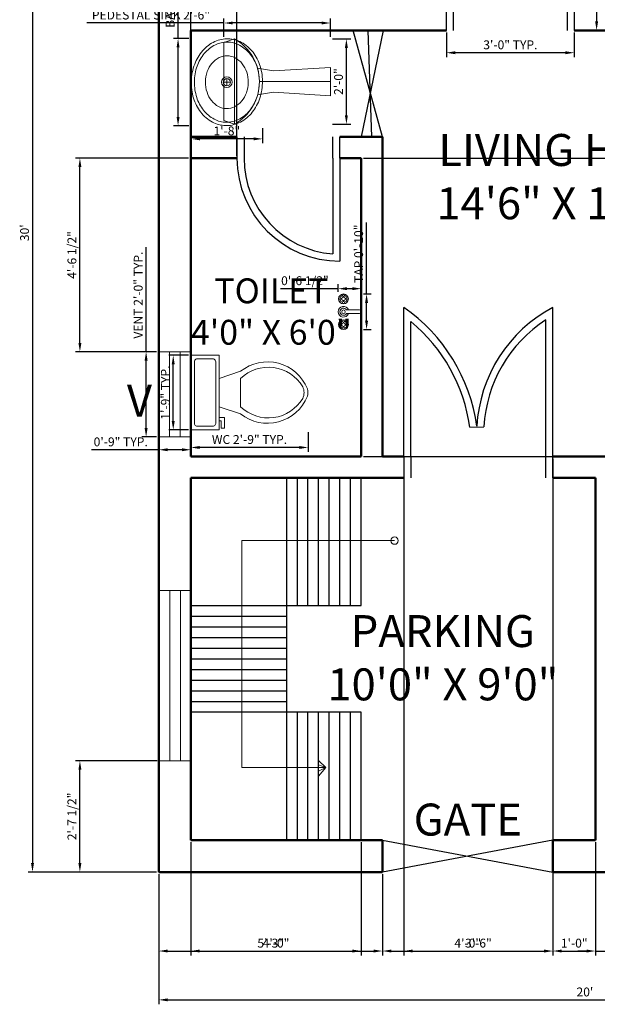
# Model space of a CAD drawing. Units: inches. Extents: x 2530 to 2846, y 1711 to 2145.
# Tile 1 of 3: x 2530 to 2693, y 1711 to 1989. Entities that reach past the tile are written whole.
import ezdxf

# ---------------------------------------------------------------- set-up
doc = ezdxf.new("R2010")
doc.units = ezdxf.units.IN
for name, color, linetype, lineweight in [('A-ANNO-DIMS', 2, 'Continuous', 18), ('A-ANNO-SYMB', 2, 'Continuous', 18), ('A-ANNO-TEXT', 7, 'Continuous', 18), ('A-AREA-IDEN', 7, 'Continuous', 25), ('A-DOOR', 3, 'Continuous', 25), ('A-FLOR-FIXT', 9, 'Continuous', 18), ('A-FLOR-STRS', 7, 'Continuous', 25), ('A-GLAZ', 4, 'Continuous', 18), ('A-WALL', 7, 'Continuous', 50)]:
    doc.layers.add(name, color=color, linetype=linetype, lineweight=lineweight)
doc.styles.get("Standard").update_dxf_attribs({"font": 'arial.ttf'})
doc.dimstyles.new('ISO-25', dxfattribs={"dimtxt": 2.5, "dimasz": 2.5, "dimexe": 1.25, "dimexo": 0.625, "dimtad": 1, "dimdec": 0, "dimlunit": 3, "dimtxsty": 'Standard', "dimcen": 2.5, "dimadec": 0, "dimazin": 0, "dimtfac": 1, "dimtdec": 0, "dimtmove": 0, "dimatfit": 3, "dimfxl": 1, "dimarcsym": 0})

# ---------------------------------------------------------------- blocks, each defined once
blk = doc.blocks.new('Faucet - Bathroom top')
for p, q in [((-4.107, 0.125), (-4.375, 0.125)), ((-3.75, 0.4788), (-3.75, 0.75)), ((-3.5, 0.482), (-3.5, 0.75)), ((-3.1461, 0.125), (-2.875, 0.125)), ((3.143, 0.125), (2.875, 0.125)), ((3.5, 0.4788), (3.5, 0.75)), ((3.75, 0.482), (3.75, 0.75)), ((4.1039, 0.125), (4.375, 0.125)), ((-4.1039, -0.125), (-4.375, -0.125)), ((-3.75, -0.4821), (-3.75, -0.75)), ((-3.5, -0.4789), (-3.5, -0.75)), ((-3.143, -0.125), (-2.875, -0.125)), ((-0.5, -0.8639), (-0.5, -4.5)), ((0.5, -4.5), (0.5, -0.8631)), ((3.1461, -0.125), (2.875, -0.125)), ((3.5, -0.4821), (3.5, -0.75)), ((3.75, -0.4789), (3.75, -0.75)), ((4.107, -0.125), (4.375, -0.125))]:
    blk.add_line(p, q)
for centre, radius in [((-3.625, 0), 1.375), ((-4.625, 0), 0.2795), ((-3.625, 0), 0.5), ((-3.625, 1), 0.2795), ((-2.625, 0), 0.2795), ((0, 0), 0.5), ((3.625, 0), 1.375), ((2.625, 0), 0.2795), ((3.625, 0), 0.5), ((3.625, 1), 0.2795), ((4.625, 0), 0.2795), ((-3.625, -1), 0.2795), ((3.625, -1), 0.2795)]:
    blk.add_circle(centre, radius)
for centre, radius, start, end in [((-3.625, 0), 1, 105.2407, 164.2093), ((-3.625, 0), 1, 16.44125, 74.07887), ((0, 0), 1.5, 289.6514, 250.3603), ((0, 0), 1, 300.3431, 239.7554), ((3.625, 0), 1, 106.12, 164.0884), ((3.625, 0), 1, 16.23422, 73.90469), ((-3.625, 0), 1, 196.2342, 253.9047), ((-3.625, 0), 1, 286.12, 344.0884), ((3.625, 0), 1, 196.4413, 254.0789), ((3.625, 0), 1, 285.2407, 344.2093), ((0, -4.5), 0.5, 180, 0)]:
    blk.add_arc(centre, radius, start, end)
blk = doc.blocks.new('Toilet - top')
for p, q in [((9.5, -6), (9.5, -2)), ((-8, -8.5), (-8, -8)), ((-7, -8), (-7, -9.5)), ((-4, -8), (-6, -14)), ((4, -8), (6, -14)), ((-10, -8.5), (-8, -8.5)), ((-10, -9.5), (-10, -8.5)), ((-7, -9.5), (-10, -9.5)), ((4, -14), (-4, -14))]:
    blk.add_line(p, q)
blk.add_lwpolyline([(10.5, -8), (10.5, 0), (-10.5, 0), (-10.5, -8)], close=True)
for points in [[(-9.5, -2), (-9.5, -6)], [(8.5, -1), (-8.5, -1)], [(-8.5, -7), (8.5, -7)]]:
    blk.add_lwpolyline(points)
for centre, radius, start, end in [((-8.62, -1.88), 0.884, 81.8699, 188.1301), ((8.62, -1.88), 0.884, 351.8699, 98.1301), ((-8.62, -6.12), 0.884, 171.8699, 278.1301), ((8.62, -6.12), 0.884, 261.8699, 8.1301), ((3.52, -21.58), 12.17, 141.4691, 247.9714), ((4.2, -21.82), 11.33, 136.3677, 238.9468), ((-3.52, -21.58), 12.17, 292.0284, 38.5307), ((-4.2, -21.82), 11.33, 301.053, 43.6321), ((0, -27.88), 4, 245.7318, 294.2682), ((0, -29), 4, 254.8605, 285.1395)]:
    blk.add_arc(centre, radius, start, end)
blk = doc.blocks.new('Sink - Oval top')
for p, q in [((-1, 0), (1, 0)), ((0, 1), (0, -1))]:
    blk.add_line(p, q)
for points in [[(-12.23, 0.39, 0.117634), (-11.46, -3.36, 0.104469), (-8.88, -6.8, 0.090016), (-5.08, -9.07, 0.08192), (-0.32, -10.02, 0.08192), (4.49, -9.38, 0.090016), (8.42, -7.36, 0.104469), (11.22, -4.09, 0.117634), (12.23, -0.39, 0.117634), (11.46, 3.36, 0.104469), (8.88, 6.8, 0.090016), (5.08, 9.07, 0.08192), (0.32, 10.02, 0.08192), (-4.49, 9.38, 0.090016), (-8.42, 7.36, 0.104469), (-11.22, 4.09, 0.117634)], [(-11.29, 0.16, 0.118622), (-10.52, -3.25, 0.104678), (-8.07, -6.36, 0.089562), (-4.54, -8.37, 0.081185), (-0.13, -9.15, 0.081185), (4.3, -8.49, 0.089562), (7.89, -6.58, 0.104678), (10.42, -3.55, 0.118622), (11.29, -0.16, 0.118622), (10.52, 3.25, 0.104678), (8.07, 6.36, 0.089562), (4.54, 8.37, 0.081185), (0.13, 9.15, 0.081185), (-4.3, 8.49, 0.089562), (-7.89, 6.58, 0.104678), (-10.42, 3.55, 0.118622)], [(-7.42, 0.08, 0.118283), (-6.91, -2.17, 0.104607), (-5.29, -4.21, 0.089718), (-2.97, -5.53, 0.081436), (-0.07, -6.04, 0.081436), (2.84, -5.59, 0.089718), (5.2, -4.33, 0.104607), (6.86, -2.32, 0.118283), (7.42, -0.08, 0.118283), (6.91, 2.17, 0.104607), (5.29, 4.21, 0.089718), (2.97, 5.53, 0.081436), (0.07, 6.04, 0.081436), (-2.84, 5.59, 0.089718), (-5.2, 4.33, 0.104607), (-6.86, 2.32, 0.118283)]]:
    blk.add_lwpolyline(points, format="xyb", close=True)
for radius in [1.5, 1]:
    blk.add_circle((0, 0), radius)
blk = doc.blocks.new('*D13')
at = {"layer": 'A-ANNO-DIMS', "color": 0, "lineweight": -2, "transparency": 16777216}
for p, q in [((2568.82, 2108.63), (2532.59, 2108.63)), ((2533.84, 2106.13), (2533.84, 1751.13)), ((2568.82, 1748.63), (2532.59, 1748.63))]:
    blk.add_line(p, q, dxfattribs=at)
at = {"layer": 'A-ANNO-DIMS', "color": 0, "transparency": 16777216}
for points in [[(2533.43, 2106.13), (2534.26, 2106.13), (2533.84, 2108.63)], [(2533.43, 1751.13), (2534.26, 1751.13), (2533.84, 1748.63)]]:
    blk.add_solid(points, dxfattribs=at)
at = {"layer": 'Defpoints', "color": 0, "transparency": 16777216}
for p in [(2569.45, 2108.63), (2533.84, 1748.63), (2569.45, 1748.63)]:
    blk.add_point(p, dxfattribs=at)
at = {"layer": 'A-ANNO-DIMS', "color": 0, "transparency": 16777216, "insert": (2531.94, 1928.63), "char_height": 2.5, "attachment_point": 5, "rotation": 90}
blk.add_mtext("30'", dxfattribs=at)
blk = doc.blocks.new('*D14')
at = {"layer": 'A-ANNO-DIMS', "color": 0, "lineweight": -2, "transparency": 16777216}
for p, q in [((2569.45, 1748), (2569.45, 1711.38)), ((2809.45, 1748), (2809.45, 1711.38)), ((2571.95, 1712.63), (2806.95, 1712.63))]:
    blk.add_line(p, q, dxfattribs=at)
at = {"layer": 'A-ANNO-DIMS', "color": 0, "transparency": 16777216}
for points in [[(2571.95, 1713.05), (2571.95, 1712.21), (2569.45, 1712.63)], [(2806.95, 1713.05), (2806.95, 1712.21), (2809.45, 1712.63)]]:
    blk.add_solid(points, dxfattribs=at)
at = {"layer": 'Defpoints', "color": 0, "transparency": 16777216}
for p in [(2569.45, 1748.63), (2809.45, 1748.63), (2809.45, 1712.63)]:
    blk.add_point(p, dxfattribs=at)
at = {"layer": 'A-ANNO-DIMS', "color": 0, "transparency": 16777216, "insert": (2689.45, 1714.53), "char_height": 2.5, "attachment_point": 5}
blk.add_mtext("20'", dxfattribs=at)
blk = doc.blocks.new('Sink - Pedestal elevation')
for p, q in [((-11, 30), (-12, 27)), ((-11, 30), (11, 30)), ((11, 30), (12, 27)), ((-12, 27), (12, 27)), ((-3, 16), (-3.7523, 20.5139)), ((0, 20), (0, 0)), ((3.7527, 20.5157), (3, 16)), ((-4, 0), (-3, 16)), ((3, 16), (4, 0)), ((-4, 0), (4, 0))]:
    blk.add_line(p, q)
blk.add_arc((0, 33.7857), 13.7857, 209.4871, 330.5129)
blk = doc.blocks.new('WIN-48IN')
for p, q in [((0, 48), (0, 0)), ((9, 48), (0, 48)), ((3, 48), (3, 0)), ((6, 0), (6, 48)), ((9, 0), (9, 48)), ((0, 0), (9, 0))]:
    blk.add_line(p, q)
blk = doc.blocks.new('VENT-24IN')
for p, q in [((24, 9), (0, 9)), ((0, 9), (0, 0)), ((24, 0), (24, 9)), ((24, 6), (0, 6)), ((0, 3), (24, 3)), ((0, 0), (24, 0))]:
    blk.add_line(p, q)
blk = doc.blocks.new('DOOR-SINGLE-29IN')
for p, q in [((0, 35), (0, 29)), ((2, 35), (2, 29)), ((27, 29), (27, 35)), ((29, 29), (29, 35)), ((27, 29), (27, 2.07)), ((29, 29), (29, 0))]:
    blk.add_line(p, q)
for radius, end in [(29, 270), (27, 265.752)]:
    blk.add_arc((29, 29), radius, 180, end)
blk = doc.blocks.new('DOOR-SINGLE-36IN')
for p, q in [((0, 36), (0, 42)), ((2, 36), (2, 42)), ((34, 42), (34, 36)), ((36, 42), (36, 36)), ((0, 36), (0, 0)), ((2, 36), (2, 2.06))]:
    blk.add_line(p, q)
for radius, start in [(36, 270), (34, 273.3723)]:
    blk.add_arc((0, 36), radius, start, 0)
blk = doc.blocks.new('*D24')
at = {"layer": 'A-ANNO-DIMS', "color": 0, "lineweight": -2, "transparency": 16777216}
for p, q in [((2578.45, 1872.51), (2578.45, 1866.92)), ((2611.49, 1872.51), (2611.49, 1866.92)), ((2608.99, 1868.17), (2580.95, 1868.17))]:
    blk.add_line(p, q, dxfattribs=at)
at = {"layer": 'A-ANNO-DIMS', "color": 0, "transparency": 16777216}
for points in [[(2580.95, 1868.59), (2580.95, 1867.76), (2578.45, 1868.17)], [(2608.99, 1868.59), (2608.99, 1867.76), (2611.49, 1868.17)]]:
    blk.add_solid(points, dxfattribs=at)
at = {"layer": 'Defpoints', "color": 0, "transparency": 16777216}
for p in [(2578.45, 1873.13), (2611.49, 1873.13), (2578.45, 1868.17)]:
    blk.add_point(p, dxfattribs=at)
at = {"layer": 'A-ANNO-DIMS', "color": 0, "transparency": 16777216, "insert": (2594.97, 1870.09), "char_height": 2.5, "attachment_point": 5}
blk.add_mtext('WC 2\'-9" TYP.', dxfattribs=at)
blk = doc.blocks.new('*D25')
at = {"layer": 'A-ANNO-DIMS', "color": 0, "lineweight": -2, "transparency": 16777216}
for p, q in [((2577.82, 1894.13), (2572.24, 1894.13)), ((2573.49, 1875.63), (2573.49, 1891.63)), ((2577.82, 1873.13), (2572.24, 1873.13))]:
    blk.add_line(p, q, dxfattribs=at)
at = {"layer": 'A-ANNO-DIMS', "color": 0, "transparency": 16777216}
for points in [[(2573.07, 1891.63), (2573.91, 1891.63), (2573.49, 1894.13)], [(2573.07, 1875.63), (2573.91, 1875.63), (2573.49, 1873.13)]]:
    blk.add_solid(points, dxfattribs=at)
at = {"layer": 'Defpoints', "color": 0, "transparency": 16777216}
for p in [(2573.49, 1894.13), (2578.45, 1894.13), (2578.45, 1873.13)]:
    blk.add_point(p, dxfattribs=at)
at = {"layer": 'A-ANNO-DIMS', "color": 0, "transparency": 16777216, "insert": (2571.59, 1883.63), "char_height": 2.5, "attachment_point": 5, "rotation": 90}
blk.add_mtext('1\'-9" TYP.', dxfattribs=at)
blk = doc.blocks.new('*D28')
at = {"layer": 'A-ANNO-DIMS', "color": 0, "lineweight": -2, "transparency": 16777216}
for p, q in [((2565.85, 1895.13), (2565.85, 1924.54)), ((2568.82, 1895.13), (2564.6, 1895.13)), ((2565.85, 1873.63), (2565.85, 1892.63)), ((2568.82, 1871.13), (2564.6, 1871.13))]:
    blk.add_line(p, q, dxfattribs=at)
at = {"layer": 'A-ANNO-DIMS', "color": 0, "transparency": 16777216}
for points in [[(2565.43, 1892.63), (2566.27, 1892.63), (2565.85, 1895.13)], [(2565.43, 1873.63), (2566.27, 1873.63), (2565.85, 1871.13)]]:
    blk.add_solid(points, dxfattribs=at)
at = {"layer": 'Defpoints', "color": 0, "transparency": 16777216}
for p in [(2565.85, 1895.13), (2569.45, 1895.13), (2569.45, 1871.13)]:
    blk.add_point(p, dxfattribs=at)
at = {"layer": 'A-ANNO-DIMS', "color": 0, "transparency": 16777216, "insert": (2563.95, 1911.08), "char_height": 2.5, "attachment_point": 5, "rotation": 90}
blk.add_mtext('VENT 2\'-0" TYP.', dxfattribs=at)
blk = doc.blocks.new('*D29')
at = {"layer": 'A-ANNO-DIMS', "color": 0, "lineweight": -2, "transparency": 16777216}
for p, q in [((2569.45, 1870.51), (2569.45, 1866.28)), ((2578.45, 1870.51), (2578.45, 1866.28)), ((2569.45, 1867.53), (2550.46, 1867.53)), ((2575.95, 1867.53), (2571.95, 1867.53))]:
    blk.add_line(p, q, dxfattribs=at)
at = {"layer": 'A-ANNO-DIMS', "color": 0, "transparency": 16777216}
for points in [[(2571.95, 1867.95), (2571.95, 1867.12), (2569.45, 1867.53)], [(2575.95, 1867.95), (2575.95, 1867.12), (2578.45, 1867.53)]]:
    blk.add_solid(points, dxfattribs=at)
at = {"layer": 'Defpoints', "color": 0, "transparency": 16777216}
for p in [(2569.45, 1871.13), (2578.45, 1871.13), (2569.45, 1867.53)]:
    blk.add_point(p, dxfattribs=at)
at = {"layer": 'A-ANNO-DIMS', "color": 0, "transparency": 16777216, "insert": (2558.7, 1869.43), "char_height": 2.5, "attachment_point": 5}
blk.add_mtext('0\'-9" TYP.', dxfattribs=at)
blk = doc.blocks.new('*D32')
at = {"layer": 'A-ANNO-DIMS', "color": 0, "lineweight": -2, "transparency": 16777216}
for p, q in [((2687.07, 2027.63), (2694, 2027.63)), ((2692.75, 2025.13), (2692.75, 1988.13)), ((2687.07, 1985.63), (2694, 1985.63))]:
    blk.add_line(p, q, dxfattribs=at)
at = {"layer": 'A-ANNO-DIMS', "color": 0, "transparency": 16777216}
for points in [[(2692.33, 2025.13), (2693.17, 2025.13), (2692.75, 2027.63)], [(2692.33, 1988.13), (2693.17, 1988.13), (2692.75, 1985.63)]]:
    blk.add_solid(points, dxfattribs=at)
at = {"layer": 'Defpoints', "color": 0, "transparency": 16777216}
for p in [(2686.45, 2027.63), (2686.45, 1985.63), (2692.75, 1985.63)]:
    blk.add_point(p, dxfattribs=at)
at = {"layer": 'A-ANNO-DIMS', "color": 0, "transparency": 16777216, "insert": (2690.83, 2006.63), "char_height": 2.5, "attachment_point": 5, "rotation": 90}
blk.add_mtext('DOOR 3\'-6" TYP.', dxfattribs=at)
blk = doc.blocks.new('*D33')
at = {"layer": 'A-ANNO-DIMS', "color": 0, "lineweight": -2, "transparency": 16777216}
for p, q in [((2650.45, 1985), (2650.45, 1978.08)), ((2686.45, 1985), (2686.45, 1978.08)), ((2683.95, 1979.33), (2652.95, 1979.33))]:
    blk.add_line(p, q, dxfattribs=at)
at = {"layer": 'A-ANNO-DIMS', "color": 0, "transparency": 16777216}
for points in [[(2652.95, 1979.75), (2652.95, 1978.91), (2650.45, 1979.33)], [(2683.95, 1979.75), (2683.95, 1978.91), (2686.45, 1979.33)]]:
    blk.add_solid(points, dxfattribs=at)
at = {"layer": 'Defpoints', "color": 0, "transparency": 16777216}
for p in [(2650.45, 1985.63), (2686.45, 1985.63), (2650.45, 1979.33)]:
    blk.add_point(p, dxfattribs=at)
at = {"layer": 'A-ANNO-DIMS', "color": 0, "transparency": 16777216, "insert": (2668.45, 1981.23), "char_height": 2.5, "attachment_point": 5}
blk.add_mtext('3\'-0" TYP.', dxfattribs=at)
blk = doc.blocks.new('*D34')
at = {"layer": 'A-ANNO-DIMS', "color": 0, "lineweight": -2, "transparency": 16777216}
for p, q in [((2627.95, 1911.39), (2627.95, 1931.55)), ((2627.07, 1911.39), (2629.2, 1911.39)), ((2627.95, 1903.89), (2627.95, 1908.89)), ((2627.07, 1901.39), (2629.2, 1901.39))]:
    blk.add_line(p, q, dxfattribs=at)
at = {"layer": 'A-ANNO-DIMS', "color": 0, "transparency": 16777216}
for points in [[(2627.53, 1908.89), (2628.37, 1908.89), (2627.95, 1911.39)], [(2627.53, 1903.89), (2628.37, 1903.89), (2627.95, 1901.39)]]:
    blk.add_solid(points, dxfattribs=at)
at = {"layer": 'Defpoints', "color": 0, "transparency": 16777216}
for p in [(2626.45, 1911.39), (2627.95, 1911.39), (2626.45, 1901.39)]:
    blk.add_point(p, dxfattribs=at)
at = {"layer": 'A-ANNO-DIMS', "color": 0, "transparency": 16777216, "insert": (2626.05, 1922.72), "char_height": 2.5, "attachment_point": 5, "rotation": 90}
blk.add_mtext('TAP 0\'-10"', dxfattribs=at)
blk = doc.blocks.new('*D35')
at = {"layer": 'A-ANNO-DIMS', "color": 0, "lineweight": -2, "transparency": 16777216}
for p, q in [((2619.95, 1912.01), (2619.95, 1914.14)), ((2626.45, 1912.01), (2626.45, 1914.14)), ((2619.95, 1912.89), (2603.73, 1912.89)), ((2623.95, 1912.89), (2622.45, 1912.89))]:
    blk.add_line(p, q, dxfattribs=at)
at = {"layer": 'A-ANNO-DIMS', "color": 0, "transparency": 16777216}
for points in [[(2622.45, 1913.31), (2622.45, 1912.47), (2619.95, 1912.89)], [(2623.95, 1913.31), (2623.95, 1912.47), (2626.45, 1912.89)]]:
    blk.add_solid(points, dxfattribs=at)
at = {"layer": 'Defpoints', "color": 0, "transparency": 16777216}
for p in [(2619.95, 1912.89), (2619.95, 1911.39), (2626.45, 1911.39)]:
    blk.add_point(p, dxfattribs=at)
at = {"layer": 'A-ANNO-DIMS', "color": 0, "transparency": 16777216, "insert": (2610.59, 1914.81), "char_height": 2.5, "attachment_point": 5}
blk.add_mtext('0\'-6 1/2"', dxfattribs=at)
blk = doc.blocks.new('*D44')
at = {"layer": 'A-ANNO-DIMS', "color": 0, "lineweight": -2, "transparency": 16777216}
for p, q in [((2574.85, 1983.31), (2574.85, 2010.87)), ((2577.91, 1983.31), (2573.6, 1983.31)), ((2574.85, 1961.26), (2574.85, 1980.81)), ((2577.91, 1958.76), (2573.6, 1958.76))]:
    blk.add_line(p, q, dxfattribs=at)
at = {"layer": 'A-ANNO-DIMS', "color": 0, "transparency": 16777216}
for points in [[(2574.43, 1980.81), (2575.27, 1980.81), (2574.85, 1983.31)], [(2574.43, 1961.26), (2575.27, 1961.26), (2574.85, 1958.76)]]:
    blk.add_solid(points, dxfattribs=at)
at = {"layer": 'Defpoints', "color": 0, "transparency": 16777216}
for p in [(2574.85, 1983.31), (2578.53, 1983.31), (2578.53, 1958.76)]:
    blk.add_point(p, dxfattribs=at)
at = {"layer": 'A-ANNO-DIMS', "color": 0, "transparency": 16777216, "insert": (2572.93, 1998.34), "char_height": 2.5, "attachment_point": 5, "rotation": 90}
blk.add_mtext('BASIN 2\'-0 1/2"', dxfattribs=at)
blk = doc.blocks.new('*D45')
at = {"layer": 'A-ANNO-DIMS', "color": 0, "lineweight": -2, "transparency": 16777216}
for p, q in [((2578.53, 1958.13), (2578.53, 1953.82)), ((2598.67, 1958.13), (2598.67, 1953.82)), ((2596.17, 1955.07), (2581.03, 1955.07))]:
    blk.add_line(p, q, dxfattribs=at)
at = {"layer": 'A-ANNO-DIMS', "color": 0, "transparency": 16777216}
for points in [[(2581.03, 1955.49), (2581.03, 1954.66), (2578.53, 1955.07)], [(2596.17, 1955.49), (2596.17, 1954.66), (2598.67, 1955.07)]]:
    blk.add_solid(points, dxfattribs=at)
at = {"layer": 'Defpoints', "color": 0, "transparency": 16777216}
for p in [(2578.53, 1958.76), (2598.67, 1958.76), (2578.53, 1955.07)]:
    blk.add_point(p, dxfattribs=at)
at = {"layer": 'A-ANNO-DIMS', "color": 0, "transparency": 16777216, "insert": (2588.6, 1956.98), "char_height": 2.5, "attachment_point": 5}
blk.add_mtext('1\'-8"', dxfattribs=at)
blk = doc.blocks.new('*D46')
at = {"layer": 'A-ANNO-DIMS', "color": 0, "lineweight": -2, "transparency": 16777216}
for p, q in [((2587.77, 1983.82), (2587.77, 1988.95)), ((2617.77, 1983.82), (2617.77, 1988.95)), ((2587.77, 1987.7), (2549.16, 1987.7)), ((2615.27, 1987.7), (2590.27, 1987.7))]:
    blk.add_line(p, q, dxfattribs=at)
at = {"layer": 'A-ANNO-DIMS', "color": 0, "transparency": 16777216}
for points in [[(2590.27, 1988.11), (2590.27, 1987.28), (2587.77, 1987.7)], [(2615.27, 1988.11), (2615.27, 1987.28), (2617.77, 1987.7)]]:
    blk.add_solid(points, dxfattribs=at)
at = {"layer": 'Defpoints', "color": 0, "transparency": 16777216}
for p in [(2587.77, 1987.7), (2587.77, 1983.2), (2617.77, 1983.2)]:
    blk.add_point(p, dxfattribs=at)
at = {"layer": 'A-ANNO-DIMS', "color": 0, "transparency": 16777216, "insert": (2567.21, 1989.62), "char_height": 2.5, "attachment_point": 5}
blk.add_mtext('PEDESTAL SINK 2\'-6"', dxfattribs=at)
blk = doc.blocks.new('*D47')
at = {"layer": 'A-ANNO-DIMS', "color": 0, "lineweight": -2, "transparency": 16777216}
for p, q in [((2618.39, 1983.2), (2623.52, 1983.2)), ((2622.27, 1961.7), (2622.27, 1980.7)), ((2618.39, 1959.2), (2623.52, 1959.2))]:
    blk.add_line(p, q, dxfattribs=at)
at = {"layer": 'A-ANNO-DIMS', "color": 0, "transparency": 16777216}
for points in [[(2621.85, 1980.7), (2622.68, 1980.7), (2622.27, 1983.2)], [(2621.85, 1961.7), (2622.68, 1961.7), (2622.27, 1959.2)]]:
    blk.add_solid(points, dxfattribs=at)
at = {"layer": 'Defpoints', "color": 0, "transparency": 16777216}
for p in [(2617.77, 1983.2), (2622.27, 1983.2), (2617.77, 1959.2)]:
    blk.add_point(p, dxfattribs=at)
at = {"layer": 'A-ANNO-DIMS', "color": 0, "transparency": 16777216, "insert": (2620.37, 1971.2), "char_height": 2.5, "attachment_point": 5, "rotation": 90}
blk.add_mtext('2\'-0"', dxfattribs=at)
blk = doc.blocks.new('*D48')
at = {"layer": 'A-ANNO-DIMS', "color": 0, "lineweight": -2, "transparency": 16777216}
for p, q in [((2569.45, 1748), (2569.45, 1725.13)), ((2632.45, 1748), (2632.45, 1725.13)), ((2571.95, 1726.38), (2629.95, 1726.38))]:
    blk.add_line(p, q, dxfattribs=at)
at = {"layer": 'A-ANNO-DIMS', "color": 0, "transparency": 16777216}
for points in [[(2571.95, 1726.8), (2571.95, 1725.96), (2569.45, 1726.38)], [(2629.95, 1726.8), (2629.95, 1725.96), (2632.45, 1726.38)]]:
    blk.add_solid(points, dxfattribs=at)
at = {"layer": 'Defpoints', "color": 0, "transparency": 16777216}
for p in [(2569.45, 1748.63), (2632.45, 1748.63), (2632.45, 1726.38)]:
    blk.add_point(p, dxfattribs=at)
at = {"layer": 'A-ANNO-DIMS', "color": 0, "transparency": 16777216, "insert": (2600.95, 1728.28), "char_height": 2.5, "attachment_point": 5}
blk.add_mtext('5\'-3"', dxfattribs=at)
blk = doc.blocks.new('*D49')
at = {"layer": 'A-ANNO-DIMS', "color": 0, "lineweight": -2, "transparency": 16777216}
for p, q in [((2632.45, 1748), (2632.45, 1725.13)), ((2680.45, 1748), (2680.45, 1725.13)), ((2634.95, 1726.38), (2677.95, 1726.38))]:
    blk.add_line(p, q, dxfattribs=at)
at = {"layer": 'A-ANNO-DIMS', "color": 0, "transparency": 16777216}
for points in [[(2634.95, 1726.8), (2634.95, 1725.96), (2632.45, 1726.38)], [(2677.95, 1726.8), (2677.95, 1725.96), (2680.45, 1726.38)]]:
    blk.add_solid(points, dxfattribs=at)
at = {"layer": 'Defpoints', "color": 0, "transparency": 16777216}
for p in [(2632.45, 1748.63), (2680.45, 1748.63), (2680.45, 1726.38)]:
    blk.add_point(p, dxfattribs=at)
at = {"layer": 'A-ANNO-DIMS', "color": 0, "transparency": 16777216, "insert": (2656.45, 1728.28), "char_height": 2.5, "attachment_point": 5}
blk.add_mtext('4\'-0"', dxfattribs=at)
blk = doc.blocks.new('*D50')
at = {"layer": 'A-ANNO-DIMS', "color": 0, "lineweight": -2, "transparency": 16777216}
for p, q in [((2692.45, 1757), (2692.45, 1725.13)), ((2680.45, 1748), (2680.45, 1725.13)), ((2682.95, 1726.38), (2689.95, 1726.38))]:
    blk.add_line(p, q, dxfattribs=at)
at = {"layer": 'A-ANNO-DIMS', "color": 0, "transparency": 16777216}
for points in [[(2682.95, 1726.8), (2682.95, 1725.96), (2680.45, 1726.38)], [(2689.95, 1726.8), (2689.95, 1725.96), (2692.45, 1726.38)]]:
    blk.add_solid(points, dxfattribs=at)
at = {"layer": 'Defpoints', "color": 0, "transparency": 16777216}
for p in [(2692.45, 1757.63), (2680.45, 1748.63), (2692.45, 1726.38)]:
    blk.add_point(p, dxfattribs=at)
at = {"layer": 'A-ANNO-DIMS', "color": 0, "transparency": 16777216, "insert": (2686.45, 1728.28), "char_height": 2.5, "attachment_point": 5}
blk.add_mtext('1\'-0"', dxfattribs=at)
blk = doc.blocks.new('*D51')
at = {"layer": 'A-ANNO-DIMS', "color": 0, "lineweight": -2, "transparency": 16777216}
for p, q in [((2638.45, 1865), (2638.45, 1725.13)), ((2680.45, 1865), (2680.45, 1725.13)), ((2640.95, 1726.38), (2677.95, 1726.38))]:
    blk.add_line(p, q, dxfattribs=at)
at = {"layer": 'A-ANNO-DIMS', "color": 0, "transparency": 16777216}
for points in [[(2640.95, 1726.8), (2640.95, 1725.96), (2638.45, 1726.38)], [(2677.95, 1726.8), (2677.95, 1725.96), (2680.45, 1726.38)]]:
    blk.add_solid(points, dxfattribs=at)
at = {"layer": 'Defpoints', "color": 0, "transparency": 16777216}
for p in [(2638.45, 1865.63), (2680.45, 1865.63), (2680.45, 1726.38)]:
    blk.add_point(p, dxfattribs=at)
at = {"layer": 'A-ANNO-DIMS', "color": 0, "transparency": 16777216, "insert": (2659.45, 1728.28), "char_height": 2.5, "attachment_point": 5}
blk.add_mtext('3\'-6"', dxfattribs=at)
blk = doc.blocks.new('*D57')
at = {"layer": 'A-ANNO-DIMS', "color": 0, "lineweight": -2, "transparency": 16777216}
for p, q in [((2692.45, 1757), (2692.45, 1725.13)), ((2698.45, 1757), (2698.45, 1725.13)), ((2689.95, 1726.38), (2687.45, 1726.38)), ((2692.45, 1726.38), (2698.45, 1726.38)), ((2700.95, 1726.38), (2711.34, 1726.38))]:
    blk.add_line(p, q, dxfattribs=at)
at = {"layer": 'A-ANNO-DIMS', "color": 0, "transparency": 16777216}
for points in [[(2689.95, 1726.8), (2689.95, 1725.96), (2692.45, 1726.38)], [(2700.95, 1726.8), (2700.95, 1725.96), (2698.45, 1726.38)]]:
    blk.add_solid(points, dxfattribs=at)
at = {"layer": 'Defpoints', "color": 0, "transparency": 16777216}
for p in [(2692.45, 1757.63), (2698.45, 1757.63), (2698.45, 1726.38)]:
    blk.add_point(p, dxfattribs=at)
at = {"layer": 'A-ANNO-DIMS', "color": 0, "transparency": 16777216, "insert": (2707.4, 1728.28), "char_height": 2.5, "attachment_point": 5}
blk.add_mtext('0\'-6"', dxfattribs=at)
blk = doc.blocks.new('*D58')
at = {"layer": 'A-ANNO-DIMS', "color": 0, "lineweight": -2, "transparency": 16777216}
for p, q in [((2627.07, 1949.63), (2832.95, 1949.63)), ((2831.7, 1868.13), (2831.7, 1947.13)), ((2627.07, 1865.63), (2832.95, 1865.63))]:
    blk.add_line(p, q, dxfattribs=at)
at = {"layer": 'A-ANNO-DIMS', "color": 0, "transparency": 16777216}
for points in [[(2831.28, 1947.13), (2832.12, 1947.13), (2831.7, 1949.63)], [(2831.28, 1868.13), (2832.12, 1868.13), (2831.7, 1865.63)]]:
    blk.add_solid(points, dxfattribs=at)
at = {"layer": 'Defpoints', "color": 0, "transparency": 16777216}
for p in [(2626.45, 1949.63), (2831.7, 1949.63), (2626.45, 1865.63)]:
    blk.add_point(p, dxfattribs=at)
at = {"layer": 'A-ANNO-DIMS', "color": 0, "transparency": 16777216, "insert": (2829.8, 1907.63), "char_height": 2.5, "attachment_point": 5, "rotation": 90}
blk.add_mtext('7\'-0"', dxfattribs=at)
blk = doc.blocks.new('*D63')
at = {"layer": 'A-ANNO-DIMS', "color": 0, "lineweight": -2, "transparency": 16777216}
for p, q in [((2568.95, 1779.94), (2545.95, 1779.94)), ((2547.2, 1751.13), (2547.2, 1777.44)), ((2568.82, 1748.63), (2545.95, 1748.63))]:
    blk.add_line(p, q, dxfattribs=at)
at = {"layer": 'A-ANNO-DIMS', "color": 0, "transparency": 16777216}
for points in [[(2546.78, 1777.44), (2547.62, 1777.44), (2547.2, 1779.94)], [(2546.78, 1751.13), (2547.62, 1751.13), (2547.2, 1748.63)]]:
    blk.add_solid(points, dxfattribs=at)
at = {"layer": 'Defpoints', "color": 0, "transparency": 16777216}
for p in [(2547.2, 1779.94), (2569.57, 1779.94), (2569.45, 1748.63)]:
    blk.add_point(p, dxfattribs=at)
at = {"layer": 'A-ANNO-DIMS', "color": 0, "transparency": 16777216, "insert": (2545.28, 1764.29), "char_height": 2.5, "attachment_point": 5, "rotation": 90}
blk.add_mtext('2\'-7 1/2"', dxfattribs=at)
blk = doc.blocks.new('*D67')
at = {"layer": 'A-ANNO-DIMS', "color": 0, "lineweight": -2, "transparency": 16777216}
for p, q in [((2578.45, 1757), (2578.45, 1725.13)), ((2626.45, 1757), (2626.45, 1725.13)), ((2580.95, 1726.38), (2623.95, 1726.38))]:
    blk.add_line(p, q, dxfattribs=at)
at = {"layer": 'A-ANNO-DIMS', "color": 0, "transparency": 16777216}
for points in [[(2580.95, 1726.8), (2580.95, 1725.96), (2578.45, 1726.38)], [(2623.95, 1726.8), (2623.95, 1725.96), (2626.45, 1726.38)]]:
    blk.add_solid(points, dxfattribs=at)
at = {"layer": 'Defpoints', "color": 0, "transparency": 16777216}
for p in [(2578.45, 1757.63), (2626.45, 1757.63), (2626.45, 1726.38)]:
    blk.add_point(p, dxfattribs=at)
at = {"layer": 'A-ANNO-DIMS', "color": 0, "transparency": 16777216, "insert": (2602.45, 1728.28), "char_height": 2.5, "attachment_point": 5}
blk.add_mtext('4\'-0"', dxfattribs=at)
blk = doc.blocks.new('*D68')
at = {"layer": 'A-ANNO-DIMS', "color": 0, "lineweight": -2, "transparency": 16777216}
for p, q in [((2578.45, 1950.25), (2578.45, 2132.13)), ((2591.45, 1950.25), (2591.45, 2132.13)), ((2580.95, 2130.88), (2588.95, 2130.88))]:
    blk.add_line(p, q, dxfattribs=at)
at = {"layer": 'A-ANNO-DIMS', "color": 0, "transparency": 16777216}
for points in [[(2580.95, 2131.3), (2580.95, 2130.46), (2578.45, 2130.88)], [(2588.95, 2131.3), (2588.95, 2130.46), (2591.45, 2130.88)]]:
    blk.add_solid(points, dxfattribs=at)
at = {"layer": 'Defpoints', "color": 0, "transparency": 16777216}
for p in [(2591.45, 2130.88), (2578.45, 1949.63), (2591.45, 1949.63)]:
    blk.add_point(p, dxfattribs=at)
at = {"layer": 'A-ANNO-DIMS', "color": 0, "transparency": 16777216, "insert": (2584.95, 2132.76), "char_height": 2.5, "attachment_point": 5}
blk.add_mtext('1\'-1"', dxfattribs=at)
blk = doc.blocks.new('*D71')
at = {"layer": 'A-ANNO-DIMS', "color": 0, "lineweight": -2, "transparency": 16777216}
for p, q in [((2577.82, 1949.63), (2545.95, 1949.63)), ((2547.2, 1897.63), (2547.2, 1947.13)), ((2568.82, 1895.13), (2545.95, 1895.13))]:
    blk.add_line(p, q, dxfattribs=at)
at = {"layer": 'A-ANNO-DIMS', "color": 0, "transparency": 16777216}
for points in [[(2546.78, 1947.13), (2547.62, 1947.13), (2547.2, 1949.63)], [(2546.78, 1897.63), (2547.62, 1897.63), (2547.2, 1895.13)]]:
    blk.add_solid(points, dxfattribs=at)
at = {"layer": 'Defpoints', "color": 0, "transparency": 16777216}
for p in [(2547.2, 1949.63), (2578.45, 1949.63), (2569.45, 1895.13)]:
    blk.add_point(p, dxfattribs=at)
at = {"layer": 'A-ANNO-DIMS', "color": 0, "transparency": 16777216, "insert": (2545.28, 1922.38), "char_height": 2.5, "attachment_point": 5, "rotation": 90}
blk.add_mtext('4\'-6 1/2"', dxfattribs=at)

msp = doc.modelspace()

# ---------------------------------------------------------------- linework, layer by layer
at = {"layer": 'A-ANNO-SYMB'}
for p, q in [((2635.84, 1841.94), (2592.81, 1841.94)), ((2592.81, 1841.94), (2592.81, 1778.06)), ((2614.45, 1778.06), (2614.45, 1780.06)), ((2614.45, 1780.06), (2614.45, 1778.06)), ((2616.45, 1778.06), (2614.45, 1780.06)), ((2614.45, 1780.06), (2616.45, 1778.06)), ((2592.81, 1778.06), (2614.45, 1778.06)), ((2616.45, 1778.06), (2614.45, 1778.78)), ((2614.45, 1778.78), (2616.45, 1778.06)), ((2614.45, 1778.06), (2616.45, 1778.06)), ((2616.45, 1778.06), (2614.45, 1775.63)), ((2614.45, 1775.63), (2616.45, 1778.06)), ((2616.45, 1778.06), (2614.45, 1777.04))]:
    msp.add_line(p, q, dxfattribs=at)
msp.add_circle((2635.84, 1841.94), 1.03, dxfattribs=at)
at = {"layer": 'A-DOOR'}
for p, q in [((2632.45, 1955.63), (2624.19, 1985.63)), ((2624.19, 1985.63), (2632.58, 1985.63)), ((2632.58, 1985.63), (2626.45, 1955.63)), ((2629.45, 1955.63), (2628.38, 1985.63)), ((2638.45, 1865.63), (2638.45, 1907.63)), ((2680.45, 1865.63), (2680.45, 1907.63)), ((2640.45, 1865.63), (2640.45, 1903.6)), ((2678.45, 1865.63), (2678.45, 1904.14)), ((2657.03, 1873.85), (2661.01, 1874.02)), ((2638.45, 1865.63), (2638.45, 1859.63)), ((2640.45, 1865.63), (2640.45, 1859.63)), ((2678.45, 1859.63), (2678.45, 1865.63)), ((2680.45, 1859.63), (2680.45, 1865.63)), ((2632.45, 1757.63), (2680.45, 1748.63)), ((2680.45, 1757.63), (2632.45, 1748.63)), ((2680.45, 1748.63), (2680.45, 1757.63))]:
    msp.add_line(p, q, dxfattribs=at)
for centre, radius, start, end in [((2610.46, 1867.39), 49.02, 7.904, 55.1845), ((2699.35, 1871.93), 40.4, 117.8998, 176.8794), ((2610.46, 1867.39), 47.02, 7.904, 50.3751), ((2699.35, 1871.93), 38.4, 122.9828, 176.8794)]:
    msp.add_arc(centre, radius, start, end, dxfattribs=at)
at = {"layer": 'A-FLOR-STRS'}
for p, q in [((2605.45, 1757.63), (2605.45, 1859.63)), ((2608.45, 1823.63), (2608.45, 1859.63)), ((2611.45, 1823.63), (2611.45, 1859.63)), ((2614.45, 1823.63), (2614.45, 1859.63)), ((2617.45, 1823.63), (2617.45, 1859.63)), ((2620.45, 1823.63), (2620.45, 1859.63)), ((2623.45, 1823.63), (2623.45, 1859.63)), ((2626.45, 1823.63), (2626.45, 1859.63)), ((2578.45, 1823.63), (2605.45, 1823.63)), ((2605.45, 1823.63), (2626.45, 1823.63)), ((2578.45, 1820.63), (2605.45, 1820.63)), ((2578.45, 1817.63), (2605.45, 1817.63)), ((2578.45, 1814.63), (2605.45, 1814.63)), ((2578.45, 1811.63), (2605.45, 1811.63)), ((2578.45, 1808.63), (2605.45, 1808.63)), ((2578.45, 1805.63), (2605.45, 1805.63)), ((2578.45, 1802.63), (2605.45, 1802.63)), ((2578.45, 1799.63), (2605.45, 1799.63)), ((2578.45, 1796.63), (2605.45, 1796.63)), ((2626.45, 1793.63), (2578.45, 1793.63)), ((2608.45, 1757.63), (2608.45, 1793.63)), ((2611.45, 1757.63), (2611.45, 1793.63)), ((2614.45, 1757.63), (2614.45, 1793.63)), ((2617.45, 1757.63), (2617.45, 1793.63)), ((2620.45, 1757.63), (2620.45, 1793.63)), ((2623.45, 1757.63), (2623.45, 1793.63)), ((2626.45, 1757.63), (2626.45, 1793.63))]:
    msp.add_line(p, q, dxfattribs=at)
at = {"layer": 'A-WALL'}
for p, q in [((2569.45, 1748.63), (2569.45, 2108.63)), ((2578.45, 1985.63), (2650.45, 1985.63)), ((2578.45, 1865.63), (2578.45, 1985.63)), ((2686.45, 1985.63), (2704.45, 1985.63)), ((2578.45, 1955.63), (2591.45, 1955.63)), ((2620.45, 1955.63), (2626.45, 1955.63)), ((2626.45, 1955.63), (2632.45, 1955.63)), ((2632.45, 1865.63), (2632.45, 1955.63)), ((2578.45, 1949.63), (2591.45, 1949.63)), ((2626.45, 1949.63), (2620.45, 1949.63)), ((2620.45, 1949.63), (2626.45, 1949.63)), ((2626.45, 1865.63), (2626.45, 1949.63)), ((2578.45, 1865.63), (2626.45, 1865.63)), ((2632.45, 1865.63), (2638.45, 1865.63)), ((2680.45, 1865.63), (2704.45, 1865.63)), ((2578.45, 1757.63), (2578.45, 1859.63)), ((2578.45, 1859.63), (2638.45, 1859.63)), ((2692.45, 1859.63), (2680.45, 1859.63)), ((2680.45, 1859.63), (2692.45, 1859.63)), ((2692.45, 1859.63), (2692.45, 1757.63)), ((2632.45, 1757.63), (2578.45, 1757.63)), ((2632.45, 1748.63), (2632.45, 1757.63)), ((2692.45, 1757.63), (2680.45, 1757.63)), ((2692.45, 1757.63), (2680.45, 1757.63)), ((2680.45, 1757.63), (2680.45, 1748.63)), ((2632.45, 1748.63), (2569.45, 1748.63)), ((2809.45, 1748.63), (2680.45, 1748.63))]:
    msp.add_line(p, q, dxfattribs=at)

# ---------------------------------------------------------------- block references
at = {"layer": 'A-DOOR', "rotation": 180}
msp.add_blockref('DOOR-SINGLE-36IN', (2686.45, 2027.63), dxfattribs=at)
at = {"layer": 'A-DOOR'}
msp.add_blockref('DOOR-SINGLE-29IN', (2591.45, 1920.63), dxfattribs=at)
at = {"layer": 'A-FLOR-FIXT', "rotation": 90}
for name, p in [('Sink - Oval top', (2588.6, 1971.03)), ('Sink - Pedestal elevation', (2617.77, 1971.2)), ('Faucet - Bathroom top', (2621.45, 1906.39)), ('Toilet - top', (2578.45, 1883.63))]:
    msp.add_blockref(name, p, dxfattribs=at)
at = {"layer": 'A-GLAZ'}
for name, p, rotation in [('VENT-24IN', (2578.45, 1871.13), 90.00000000000024), ('WIN-48IN', (2578.57, 1827.94), 180)]:
    msp.add_blockref(name, p, dxfattribs=dict(at, rotation=rotation))

# ---------------------------------------------------------------- texts
at = {"layer": 'A-ANNO-TEXT', "char_height": 9, "attachment_point": 1}
for s, width, insert in [('\\pxqc;V', 62.3253, (2532.8, 1885.87)), ('\\pxqc;GATE', 19.7452, (2646.6, 1767.9))]:
    msp.add_mtext_dynamic_manual_height_columns(s, width=width, gutter_width=12.5, heights=[0], dxfattribs=dict(at, insert=insert))
at = {"layer": 'A-AREA-IDEN', "attachment_point": 1}
for s, width, insert, char_height in [('\\pxqc;LIVING HALL\\P14\'6" X 10\'0"', 87.9878, (2639.57, 1956.44), 9), ('\\pxqc;TOILET\\P4\'0" X 6\'0"', 51.1196, (2575.58, 1915.78), 7), ('\\pxqc;PARKING\\P10\'0" X 9\'0"', 87.9878, (2605.45, 1820.97), 9)]:
    msp.add_mtext_dynamic_manual_height_columns(s, width=width, gutter_width=12.5, heights=[0], dxfattribs=dict(at, insert=insert, char_height=char_height))

# ---------------------------------------------------------------- dimensions: what is measured, and where the dimension line sits
at = {"layer": 'A-ANNO-DIMS'}
for base, p1, p2, override, picture, middle in [((2591.45, 2130.88), (2578.45, 1949.63), (2591.45, 1949.63), {"dimdec": 1, "dimlfac": 1, "dimrnd": 0, "dimzin": 1, "dimdsep": 46, "dimlunit": 4, "dimfrac": 2}, '*D68', (2584.95, 2132.76)), ((2680.45, 1726.38), (2638.45, 1865.63), (2680.45, 1865.63), {"dimdec": 1, "dimlfac": 1, "dimrnd": 0, "dimzin": 1, "dimdsep": 46, "dimlunit": 4, "dimfrac": 2}, '*D51', (2659.45, 1728.28)), ((2626.45, 1726.38), (2578.45, 1757.63), (2626.45, 1757.63), {"dimdec": 1, "dimlfac": 1, "dimrnd": 0, "dimzin": 1, "dimdsep": 46, "dimlunit": 4, "dimfrac": 2}, '*D67', (2602.45, 1728.28)), ((2692.45, 1726.38), (2680.45, 1748.63), (2692.45, 1757.63), {"dimdec": 1, "dimlfac": 1, "dimrnd": 0, "dimzin": 1, "dimdsep": 46, "dimlunit": 4, "dimfrac": 2}, '*D50', (2686.45, 1728.28)), ((2698.45, 1726.38), (2692.45, 1757.63), (2698.45, 1757.63), {"dimdec": 1, "dimlfac": 1, "dimrnd": 0, "dimzin": 1, "dimdsep": 46, "dimlunit": 4, "dimfrac": 2}, '*D57', (2707.4, 1728.28)), ((2809.45, 1712.63), (2569.45, 1748.63), (2809.45, 1748.63), {"dimclrd": 0, "dimclre": 0, "dimclrt": 0}, '*D14', (2689.45, 1714.53)), ((2632.45, 1726.38), (2569.45, 1748.63), (2632.45, 1748.63), {"dimdec": 1, "dimlfac": 1, "dimrnd": 0, "dimzin": 1, "dimdsep": 46, "dimlunit": 4, "dimfrac": 2}, '*D48', (2600.95, 1728.28)), ((2680.45, 1726.38), (2632.45, 1748.63), (2680.45, 1748.63), {"dimdec": 1, "dimlfac": 1, "dimrnd": 0, "dimzin": 1, "dimdsep": 46, "dimlunit": 4, "dimfrac": 2}, '*D49', (2656.45, 1728.28))]:
    dim = msp.add_linear_dim(base=base, p1=p1, p2=p2, dimstyle='ISO-25', override=override, dxfattribs=at)
    dim.commit()
    dim.dimension.update_dxf_attribs({"geometry": picture, "text_midpoint": middle})
for base, p1, p2, angle, override, picture, middle in [((2533.84, 1748.63), (2569.45, 2108.63), (2569.45, 1748.63), 90, {"dimclrd": 0, "dimclre": 0, "dimclrt": 0}, '*D13', (2531.94, 1928.63)), ((2622.27, 1983.2), (2617.77, 1959.2), (2617.77, 1983.2), 90, {"dimdec": 1, "dimlfac": 1, "dimrnd": 0, "dimzin": 1, "dimdsep": 46, "dimlunit": 4, "dimfrac": 2}, '*D47', (2620.37, 1971.2)), ((2578.53, 1955.07), (2598.67, 1958.76), (2578.53, 1958.76), 180, {"dimdec": 1, "dimlfac": 1, "dimrnd": 0, "dimzin": 1, "dimdsep": 46, "dimlunit": 4, "dimfrac": 2}, '*D45', (2588.6, 1956.98)), ((2547.2, 1949.63), (2569.45, 1895.13), (2578.45, 1949.63), 90, {"dimdec": 1, "dimlfac": 1, "dimrnd": 0, "dimzin": 1, "dimdsep": 46, "dimlunit": 4, "dimfrac": 2}, '*D71', (2545.28, 1922.38)), ((2831.7, 1949.63), (2626.45, 1865.63), (2626.45, 1949.63), 90, {"dimdec": 1, "dimlfac": 1, "dimrnd": 0, "dimzin": 1, "dimdsep": 46, "dimlunit": 4, "dimfrac": 2}, '*D58', (2829.8, 1907.63)), ((2619.95, 1912.89), (2626.45, 1911.39), (2619.95, 1911.39), 180, {"dimdec": 1, "dimlfac": 1, "dimrnd": 0, "dimzin": 1, "dimdsep": 46, "dimlunit": 4, "dimfrac": 2}, '*D35', (2610.59, 1914.81)), ((2547.2, 1779.94), (2569.45, 1748.63), (2569.57, 1779.94), 90, {"dimdec": 1, "dimlfac": 1, "dimrnd": 0, "dimzin": 1, "dimdsep": 46, "dimlunit": 4, "dimfrac": 2}, '*D63', (2545.28, 1764.29))]:
    dim = msp.add_linear_dim(base=base, p1=p1, p2=p2, angle=angle, dimstyle='ISO-25', override=override, dxfattribs=at)
    dim.commit()
    dim.dimension.update_dxf_attribs({"geometry": picture, "text_midpoint": middle})
for base, p1, p2, angle, text, picture, middle in [((2692.75, 1985.63), (2686.45, 2027.63), (2686.45, 1985.63), 270, 'DOOR <> TYP.', '*D32', (2690.83, 2006.63)), ((2574.8501, 1983.3076), (2578.5327, 1958.7567), (2578.5327, 1983.3076), 90, 'BASIN <>', '*D44', (2572.9325, 1998.3382)), ((2587.77, 1987.7), (2617.77, 1983.2), (2587.77, 1983.2), 180, 'PEDESTAL SINK <>', '*D46', (2567.21, 1989.62)), ((2650.45, 1979.33), (2686.45, 1985.63), (2650.45, 1985.63), 180, '<> TYP.', '*D33', (2668.45, 1981.23)), ((2627.95, 1911.39), (2626.45, 1901.39), (2626.45, 1911.39), 90, 'TAP <>', '*D34', (2626.05, 1922.72)), ((2565.85, 1895.13), (2569.45, 1871.13), (2569.45, 1895.13), 90, 'VENT <> TYP.', '*D28', (2563.95, 1911.08)), ((2573.49, 1894.13), (2578.45, 1873.13), (2578.45, 1894.13), 90, '<> TYP.', '*D25', (2571.59, 1883.63)), ((2578.45, 1868.17), (2611.49, 1873.13), (2578.45, 1873.13), 180, 'WC <> TYP.', '*D24', (2594.97, 1870.09)), ((2569.45, 1867.53), (2578.45, 1871.13), (2569.45, 1871.13), 180, '<> TYP.', '*D29', (2558.7, 1869.43))]:
    dim = msp.add_linear_dim(base=base, p1=p1, p2=p2, angle=angle, text=text, dimstyle='ISO-25', override={"dimdec": 1, "dimlfac": 1, "dimrnd": 0, "dimzin": 1, "dimdsep": 46, "dimlunit": 4, "dimfrac": 2}, dxfattribs=at)
    dim.commit()
    dim.dimension.update_dxf_attribs({"geometry": picture, "text_midpoint": middle})

doc.saveas('drawing.dxf')
